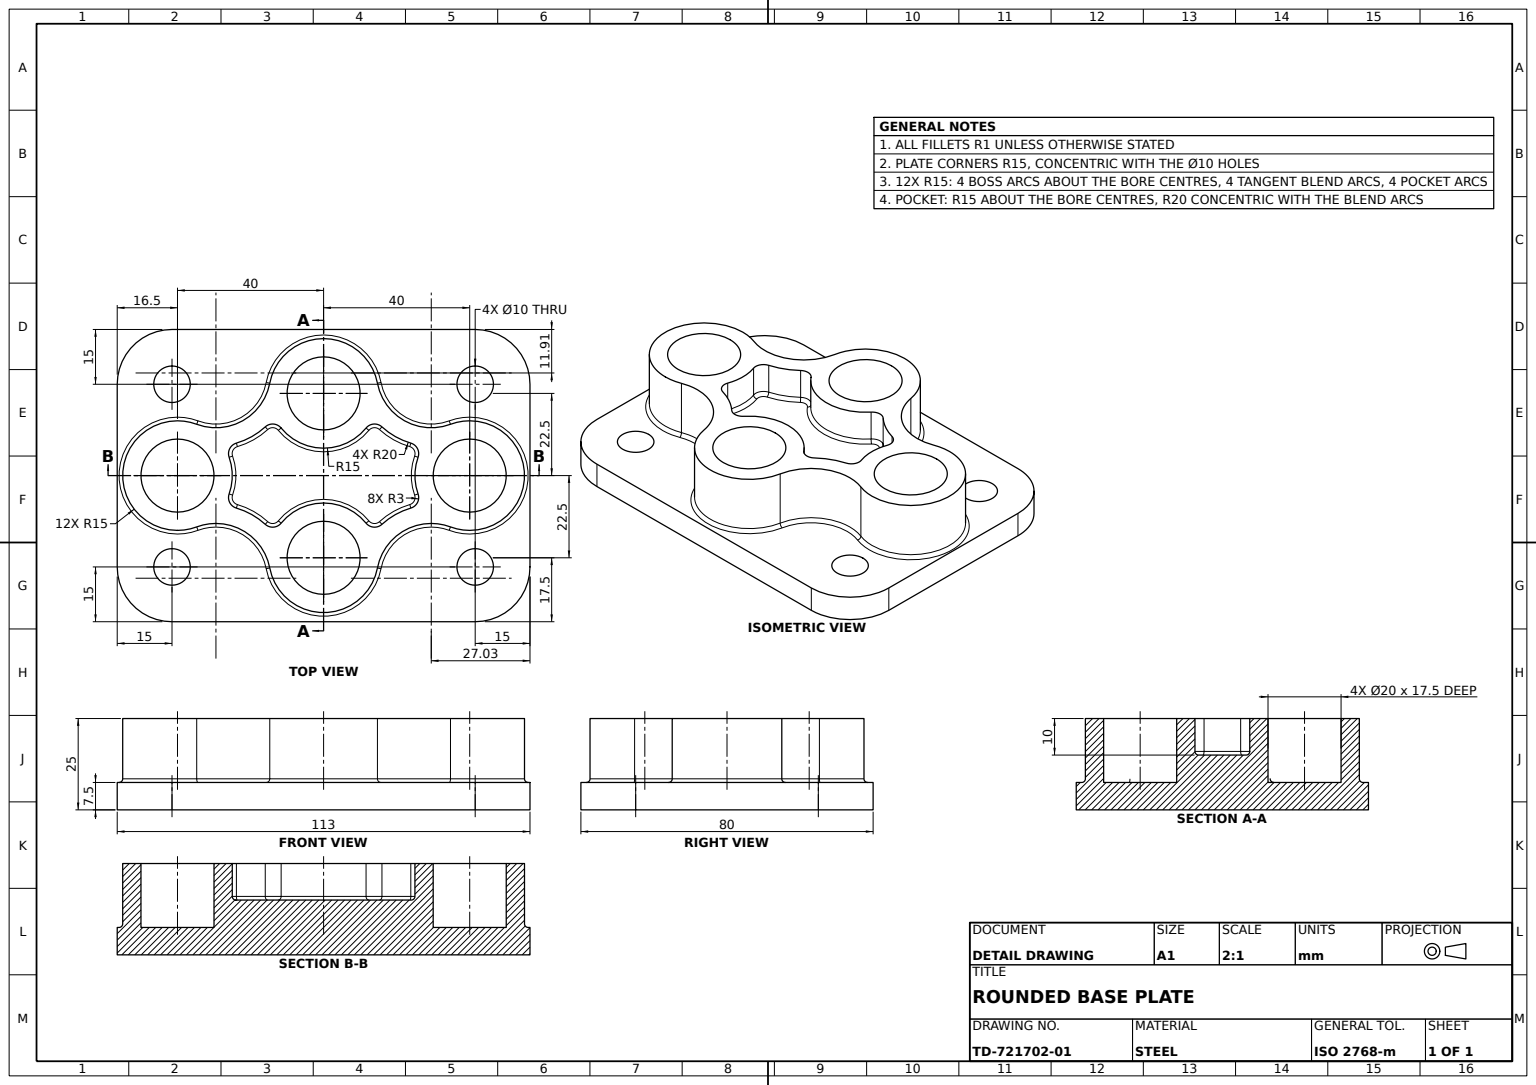
from build123d import *

# Parameters (mm, degrees)
BASE_PLATE_SKETCH_W         = 113
BASE_PLATE_SKETCH_H         = 80
BASE_PLATE_113X80X7_5_DEPTH = 7.5
QUAD_BOSS_PROFILE_SKETCH_R  = 10
QUAD_BOSS_BODY_H17_5_DEPTH  = 17.5
BOSS_ROOT_FILLET_R1_R       = 1
PLATE_CORNER_FILLETS_R15_R  = 15
BORE_CUT_SKETCH_R           = 5
BORE_CUTS_D17_5_DEPTH       = 17.5
BOSS_WEB_H7_5_DEPTH         = 7.5
WEB_BLEND_FILLET_R1_R       = 1


with BuildPart() as part:
    # Base Plate Sketch → Base Plate 113x80x7.5 (new body)
    with BuildSketch(Plane(origin=(0, 0, 0), x_dir=(1, 0, 0), z_dir=(0, 1, 0))):
        Rectangle(BASE_PLATE_SKETCH_W, BASE_PLATE_SKETCH_H)
    extrude(amount=-BASE_PLATE_113X80X7_5_DEPTH)

    # Quad Boss Profile Sketch → Quad Boss Body H17.5 (add)
    with BuildSketch(Plane(origin=(0, 0, 0), x_dir=(1, 0, 0), z_dir=(0, 1, 0))):
        with BuildLine():
            ThreePointArc((-34.737034272, 14.046394261), (-55, 0), (-34.737034272, -14.046394261))
            ThreePointArc((-34.737034272, -14.046394261), (-22.12014995, -15.019155466), (-14.737034272, -25.296394261))
            ThreePointArc((-14.737034272, -25.296394261), (0, -37.5), (14.737034272, -25.296394261))
            ThreePointArc((14.737034272, -25.296394261), (22.12014995, -15.019155466), (34.737034272, -14.046394261))
            ThreePointArc((34.737034272, -14.046394261), (55, 0), (34.737034272, 14.046394261))
            ThreePointArc((34.737034272, 14.046394261), (22.12014995, 15.019155466), (14.737034272, 25.296394261))
            ThreePointArc((14.737034272, 25.296394261), (0, 37.5), (-14.737034272, 25.296394261))
            ThreePointArc((-14.737034272, 25.296394261), (-22.12014995, 15.019155466), (-34.737034272, 14.046394261))
        make_face()
        with Locations(Location((-40, 0, 0), (0, 0, 270))):
            Circle(QUAD_BOSS_PROFILE_SKETCH_R, mode=Mode.SUBTRACT)
        with Locations(Location((0, -22.5, 0), (0, 0, 270))):
            Circle(QUAD_BOSS_PROFILE_SKETCH_R, mode=Mode.SUBTRACT)
        with Locations(Location((40, 0, 0), (0, 0, 90))):
            Circle(QUAD_BOSS_PROFILE_SKETCH_R, mode=Mode.SUBTRACT)
        with Locations(Location((0, 22.5, 0), (0, 0, 90))):
            Circle(QUAD_BOSS_PROFILE_SKETCH_R, mode=Mode.SUBTRACT)
        with BuildLine():
            ThreePointArc((25.861644904, -5.01068011), (25, 0), (25.861644904, 5.01068011))
            ThreePointArc((25.861644904, 5.01068011), (25.704313442, 7.380034713), (23.873986231, 8.892812531))
            ThreePointArc((23.873986231, 8.892812531), (19.668843751, 10.66127778), (15.97383507, 13.336647559))
            ThreePointArc((15.97383507, 13.336647559), (13.730549392, 14.115276991), (11.62400004, 13.019355346))
            ThreePointArc((11.62400004, 13.019355346), (0, 7.5), (-11.62400004, 13.019355346))
            ThreePointArc((-11.62400004, 13.019355346), (-13.730549392, 14.115276991), (-15.97383507, 13.336647559))
            ThreePointArc((-15.97383507, 13.336647559), (-19.668843751, 10.66127778), (-23.873986231, 8.892812531))
            ThreePointArc((-23.873986231, 8.892812531), (-25.704313442, 7.380034713), (-25.861644904, 5.01068011))
            ThreePointArc((-25.861644904, 5.01068011), (-25, 0), (-25.861644904, -5.01068011))
            ThreePointArc((-25.861644904, -5.01068011), (-25.704313442, -7.380034713), (-23.873986231, -8.892812531))
            ThreePointArc((-23.873986231, -8.892812531), (-19.668843751, -10.66127778), (-15.97383507, -13.336647559))
            ThreePointArc((-15.97383507, -13.336647559), (-13.730549392, -14.115276991), (-11.62400004, -13.019355346))
            ThreePointArc((-11.62400004, -13.019355346), (0, -7.5), (11.62400004, -13.019355346))
            ThreePointArc((11.62400004, -13.019355346), (13.730549392, -14.115276991), (15.97383507, -13.336647559))
            ThreePointArc((15.97383507, -13.336647559), (19.668843751, -10.66127778), (23.873986231, -8.892812531))
            ThreePointArc((23.873986231, -8.892812531), (25.704313442, -7.380034713), (25.861644904, -5.01068011))
        make_face(mode=Mode.SUBTRACT)
    extrude(amount=QUAD_BOSS_BODY_H17_5_DEPTH)

    # Boss Root Fillet R1
    boss_root_fillet_r1_edges = [part.edges().sort_by_distance(p)[0] for p in [
        (-22.12014995, 0, 15.019155466),
        (0, 0, 37.5),
        (22.12014995, 0, 15.019155466),
        (55, 0, 0),
        (22.12014995, 0, -15.019155466),
        (0, 0, -37.5),
        (-22.12014995, 0, -15.019155466),
        (-55, 0, 0),
    ]]
    fillet(boss_root_fillet_r1_edges, radius=BOSS_ROOT_FILLET_R1_R)

    # Plate Corner Fillets R15
    plate_corner_fillets_r15_edges = [part.edges().sort_by_distance(p)[0] for p in [
        (56.5, -3.75, 40),
        (-56.5, -3.75, 40),
        (-56.5, -3.75, -40),
        (56.5, -3.75, -40),
    ]]
    fillet(plate_corner_fillets_r15_edges, radius=PLATE_CORNER_FILLETS_R15_R)

    # Bore Cut Sketch → Bore Cuts D17.5 (cut)
    with BuildSketch(Plane(origin=(0, 0, 0), x_dir=(1, 0, 0), z_dir=(0, 1, 0))):
        with Locations(Location((-41.5, 25, 0), (0, 0, 270))):
            Circle(BORE_CUT_SKETCH_R)
        with Locations(Location((-41.5, -25, 0), (0, 0, 270))):
            Circle(BORE_CUT_SKETCH_R)
        with Locations(Location((41.5, -25, 0), (0, 0, 90))):
            Circle(BORE_CUT_SKETCH_R)
        with Locations(Location((41.5, 25, 0), (0, 0, 90))):
            Circle(BORE_CUT_SKETCH_R)
    extrude(amount=-BORE_CUTS_D17_5_DEPTH, mode=Mode.SUBTRACT)

    # Boss Web Offset Sketch → Boss Web H7.5 (add)
    with BuildSketch(Plane(origin=(0, 0, 0), x_dir=(1, 0, 0), z_dir=(0, 1, 0))):
        with BuildLine():
            ThreePointArc((-15.97383507, -13.336647559), (-13.730549392, -14.115276991), (-11.62400004, -13.019355346))
            ThreePointArc((-11.62400004, -13.019355346), (0, -7.5), (11.62400004, -13.019355346))
            ThreePointArc((11.62400004, -13.019355346), (13.730549392, -14.115276991), (15.97383507, -13.336647559))
            ThreePointArc((15.97383507, -13.336647559), (19.668843751, -10.66127778), (23.873986231, -8.892812531))
            ThreePointArc((23.873986231, -8.892812531), (25.704313442, -7.380034713), (25.861644904, -5.01068011))
            ThreePointArc((25.861644904, -5.01068011), (25, 0), (25.861644904, 5.01068011))
            ThreePointArc((25.861644904, 5.01068011), (25.704313442, 7.380034713), (23.873986231, 8.892812531))
            ThreePointArc((23.873986231, 8.892812531), (19.668843751, 10.66127778), (15.97383507, 13.336647559))
            ThreePointArc((15.97383507, 13.336647559), (13.730549392, 14.115276991), (11.62400004, 13.019355346))
            ThreePointArc((11.62400004, 13.019355346), (0, 7.5), (-11.62400004, 13.019355346))
            ThreePointArc((-11.62400004, 13.019355346), (-13.730549392, 14.115276991), (-15.97383507, 13.336647559))
            ThreePointArc((-15.97383507, 13.336647559), (-19.668843751, 10.66127778), (-23.873986231, 8.892812531))
            ThreePointArc((-23.873986231, 8.892812531), (-25.704313442, 7.380034713), (-25.861644904, 5.01068011))
            ThreePointArc((-25.861644904, 5.01068011), (-25, 0), (-25.861644904, -5.01068011))
            ThreePointArc((-25.861644904, -5.01068011), (-25.704313442, -7.380034713), (-23.873986231, -8.892812531))
            ThreePointArc((-23.873986231, -8.892812531), (-19.668843751, -10.66127778), (-15.97383507, -13.336647559))
        make_face()
    extrude(amount=BOSS_WEB_H7_5_DEPTH)

    # Web Blend Fillet R1
    web_blend_fillet_r1_edges = [part.edges().sort_by_distance(p)[0] for p in [
        (-19.668843751, 7.5, 10.66127778),
        (-13.730549392, 7.5, 14.115276991),
        (0, 7.5, 7.5),
        (13.730549392, 7.5, 14.115276991),
        (19.668843751, 7.5, 10.66127778),
        (25.704313442, 7.5, 7.380034713),
        (25, 7.5, 0),
        (25.704313442, 7.5, -7.380034713),
        (19.668843751, 7.5, -10.66127778),
        (13.730549392, 7.5, -14.115276991),
        (0, 7.5, -7.5),
        (-13.730549392, 7.5, -14.115276991),
        (-19.668843751, 7.5, -10.66127778),
        (-25.704313442, 7.5, -7.380034713),
        (-25, 7.5, 0),
        (-25.704313442, 7.5, 7.380034713),
    ]]
    fillet(web_blend_fillet_r1_edges, radius=WEB_BLEND_FILLET_R1_R)


solid = part.part
